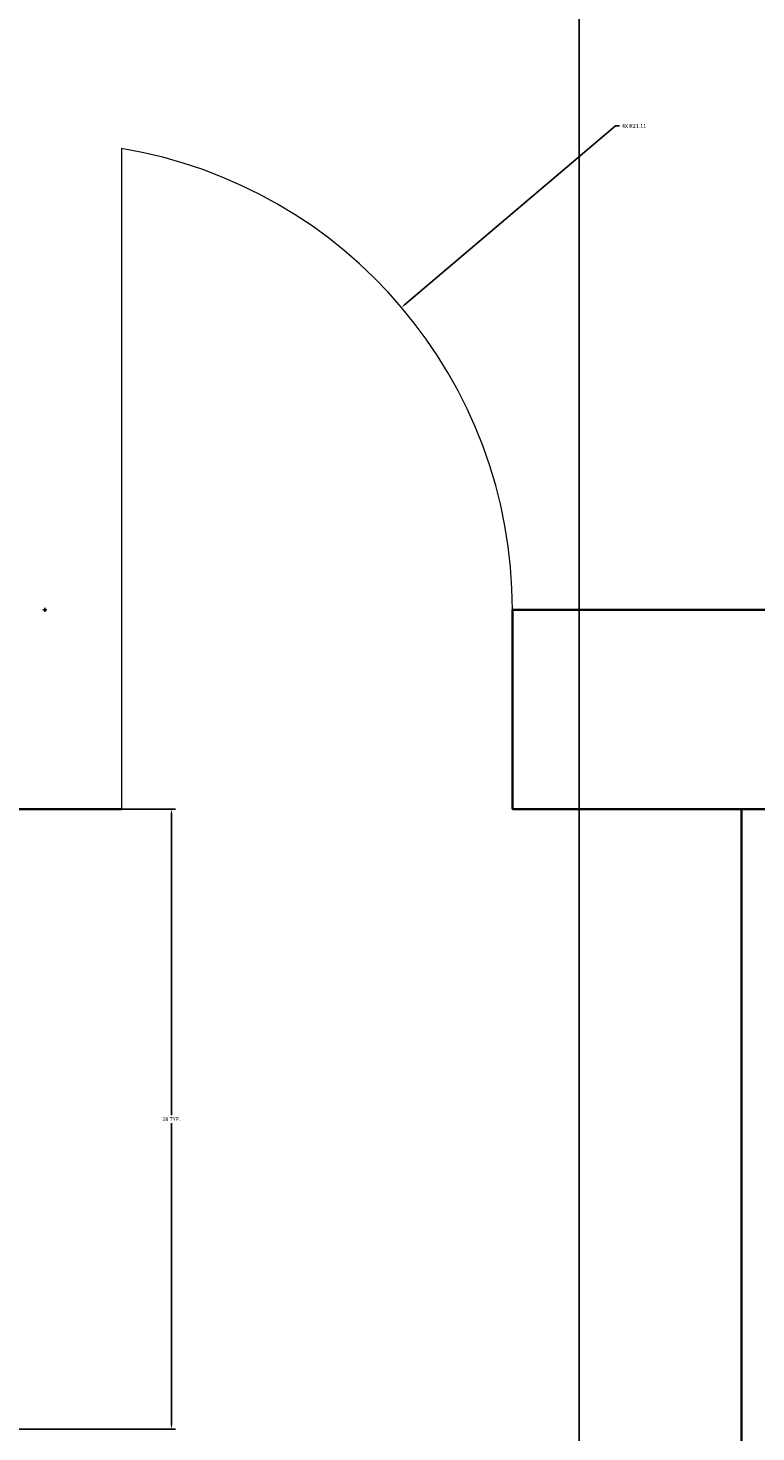
# Model space of a CAD drawing. Units: feet. Extents: x 5816 to 6644, y 25475 to 26788.
# Tile 18 of 23: x 6082 to 6115, y 26530 to 26594. Entities that reach past the tile are written whole.
import ezdxf

# ---------------------------------------------------------------- set-up
doc = ezdxf.new("R2010")
doc.units = ezdxf.units.FT
for name, color, linetype, lineweight in [('A-ANNO-DIMS', 2, 'Continuous', 13), ('A-DOOR', 3, 'Continuous', 18), ('A-WALL', 7, 'Continuous', 35)]:
    doc.layers.add(name, color=color, linetype=linetype, lineweight=lineweight)
doc.styles.get("Standard").update_dxf_attribs({"font": 'arial.ttf'})
doc.dimstyles.get("Standard").update_dxf_attribs({"dimtxt": 0.18, "dimasz": 0.18, "dimexe": 0.18, "dimexo": 0.0625, "dimgap": 0.09, "dimtad": 0, "dimtih": 1, "dimtoh": 1, "dimdec": 4, "dimzin": 0, "dimdsep": 46, "dimtxsty": 'Standard', "dimcen": 0.09, "dimadec": 0, "dimazin": 0, "dimtfac": 1, "dimtdec": 4, "dimtofl": 0, "dimtmove": 0, "dimatfit": 3, "dimfxl": 1, "dimtolj": 1, "dimtzin": 0, "dimarcsym": 0})

# ---------------------------------------------------------------- blocks, each defined once
blk = doc.blocks.new('DOOR-BEDROOM-INNER')
blk.add_line((0, 29.824), (0, 0))
blk.add_arc((-3.451, 9), 21.108, 0, 80.59123)
blk = doc.blocks.new('*D24')
at = {"layer": 'A-ANNO-DIMS', "color": 0, "lineweight": -2, "transparency": 16777216}
for p, q in [((6081.374, 26558.585), (6088.754, 26558.585)), ((6088.574, 26558.405), (6088.574, 26544.766)), ((6088.574, 26530.763), (6088.574, 26544.402)), ((6081.374, 26530.583), (6088.754, 26530.583))]:
    blk.add_line(p, q, dxfattribs=at)
at = {"layer": 'A-ANNO-DIMS', "color": 0, "transparency": 16777216}
for points in [[(6088.544, 26558.405), (6088.604, 26558.405), (6088.574, 26558.585)], [(6088.544, 26530.763), (6088.604, 26530.763), (6088.574, 26530.583)]]:
    blk.add_solid(points, dxfattribs=at)
at = {"layer": 'Defpoints', "color": 0, "transparency": 16777216}
for p in [(6081.312, 26558.585), (6088.574, 26558.585), (6081.312, 26530.583)]:
    blk.add_point(p, dxfattribs=at)
at = {"layer": 'A-ANNO-DIMS', "color": 0, "transparency": 16777216, "insert": (6088.574, 26544.584), "char_height": 0.18, "attachment_point": 5}
blk.add_mtext('\\A1;28 TYP.', dxfattribs=at)
blk = doc.blocks.new('*D58')
at = {"layer": 'A-ANNO-DIMS', "color": 0, "lineweight": -2, "transparency": 16777216}
for p, q in [((5953.978, 26168.647), (5953.978, 26787.915)), ((5954.158, 26787.735), (6030.198, 26787.735)), ((6106.798, 26787.735), (6030.759, 26787.735)), ((6106.978, 26168.713), (6106.978, 26787.915))]:
    blk.add_line(p, q, dxfattribs=at)
at = {"layer": 'A-ANNO-DIMS', "color": 0, "transparency": 16777216}
for points in [[(5954.158, 26787.765), (5954.158, 26787.705), (5953.978, 26787.735)], [(6106.798, 26787.765), (6106.798, 26787.705), (6106.978, 26787.735)]]:
    blk.add_solid(points, dxfattribs=at)
at = {"layer": 'Defpoints', "color": 0, "transparency": 16777216}
for p in [(6106.978, 26787.735), (5953.978, 26168.585), (6106.978, 26168.651)]:
    blk.add_point(p, dxfattribs=at)
at = {"layer": 'A-ANNO-DIMS', "color": 0, "transparency": 16777216, "insert": (6030.478, 26787.735), "char_height": 0.18, "attachment_point": 5}
blk.add_mtext('\\A1;153', dxfattribs=at)
blk = doc.blocks.new('*D60')
at = {"layer": 'A-ANNO-DIMS', "color": 0, "lineweight": -2, "transparency": 16777216}
for p, q in [((6106.978, 26094.399), (6106.978, 26787.915)), ((6107.158, 26787.735), (6224.932, 26787.735)), ((6343.496, 26787.735), (6225.722, 26787.735)), ((6343.676, 26094.399), (6343.676, 26787.915))]:
    blk.add_line(p, q, dxfattribs=at)
at = {"layer": 'A-ANNO-DIMS', "color": 0, "transparency": 16777216}
for points in [[(6107.158, 26787.765), (6107.158, 26787.705), (6106.978, 26787.735)], [(6343.496, 26787.765), (6343.496, 26787.705), (6343.676, 26787.735)]]:
    blk.add_solid(points, dxfattribs=at)
at = {"layer": 'Defpoints', "color": 0, "transparency": 16777216}
for p in [(6343.676, 26787.735), (6106.978, 26094.337), (6343.676, 26094.337)]:
    blk.add_point(p, dxfattribs=at)
at = {"layer": 'A-ANNO-DIMS', "color": 0, "transparency": 16777216, "insert": (6225.327, 26787.735), "char_height": 0.18, "attachment_point": 5}
blk.add_mtext('\\A1;236.7', dxfattribs=at)
blk = doc.blocks.new('*D81')
at = {"layer": 'A-ANNO-DIMS', "color": 0, "lineweight": -2, "transparency": 16777216}
for p, q in [((6108.621, 26589.427), (6099.098, 26581.353)), ((6108.801, 26589.427), (6108.621, 26589.427)), ((6082.772, 26567.585), (6082.952, 26567.585)), ((6082.862, 26567.495), (6082.862, 26567.675))]:
    blk.add_line(p, q, dxfattribs=at)
at = {"layer": 'A-ANNO-DIMS', "color": 0, "transparency": 16777216}
blk.add_solid([(6099.079, 26581.375), (6099.118, 26581.33), (6098.961, 26581.236)], dxfattribs=at)
at = {"layer": 'Defpoints', "color": 0, "transparency": 16777216}
for p in [(6098.961, 26581.236), (6082.862, 26567.585)]:
    blk.add_point(p, dxfattribs=at)
at = {"layer": 'A-ANNO-DIMS', "color": 0, "transparency": 16777216, "insert": (6109.46, 26589.427), "char_height": 0.18, "attachment_point": 5}
blk.add_mtext('\\A1;4X R21.11', dxfattribs=at)

msp = doc.modelspace()

# ---------------------------------------------------------------- linework, layer by layer
at = {"layer": 'A-WALL'}
for p, q in [((6103.9699, 26567.5846), (6103.9699, 26558.5846)), ((6127.6877, 26567.5846), (6103.9699, 26567.5846)), ((6086.3125, 26558.5846), (6072.3119, 26558.5846)), ((6127.6877, 26558.5846), (6103.9699, 26558.5846)), ((6114.3119, 26558.5846), (6114.3119, 26491.3288))]:
    msp.add_line(p, q, dxfattribs=at)

# ---------------------------------------------------------------- block references
at = {"layer": 'A-DOOR'}
msp.add_blockref('DOOR-BEDROOM-INNER', (6086.3125, 26558.5846), dxfattribs=at)

# ---------------------------------------------------------------- dimensions: what is measured, and where the dimension line sits
at = {"layer": 'A-ANNO-DIMS'}
for base, p1, p2, override, picture, middle in [((6106.9781, 26787.7346), (5953.9781, 26168.5846), (6106.9781, 26168.6509), {"dimdec": 0, "dimlfac": 1, "dimrnd": 0, "dimzin": 0, "dimdsep": 46, "dimlunit": 2}, '*D58', (6030.4781, 26787.7346)), ((6343.6763, 26787.7346), (6106.9781, 26094.3368), (6343.6763, 26094.3368), {"dimdec": 1, "dimlfac": 1, "dimrnd": 0, "dimzin": 0, "dimdsep": 46, "dimlunit": 2}, '*D60', (6225.3272, 26787.7346))]:
    dim = msp.add_linear_dim(base=base, p1=p1, p2=p2, dimstyle='Standard', override=override, dxfattribs=at)
    dim.commit()
    dim.dimension.update_dxf_attribs({"geometry": picture, "text_midpoint": middle})
dim = msp.add_radius_dim(center=(6082.8618, 26567.5846), mpoint=(6098.9612, 26581.2361), text='4X <>', dimstyle='Standard', override={"dimdec": 2, "dimlfac": 1, "dimrnd": 0, "dimzin": 0, "dimdsep": 46, "dimlunit": 2}, dxfattribs=at)
dim.commit()
dim.dimension.update_dxf_attribs({"geometry": '*D81', "text_midpoint": (6109.4603, 26589.4271), "dimtype": 164})
dim = msp.add_linear_dim(base=(6088.5736, 26558.5846), p1=(6081.3119, 26530.5827), p2=(6081.3119, 26558.5846), angle=90, text='<> TYP.', dimstyle='Standard', override={"dimdec": 0, "dimlfac": 1, "dimrnd": 0, "dimzin": 0, "dimdsep": 46, "dimlunit": 2}, dxfattribs=at)
dim.commit()
dim.dimension.update_dxf_attribs({"geometry": '*D24', "text_midpoint": (6088.5736, 26544.5837)})

doc.saveas('drawing.dxf')
